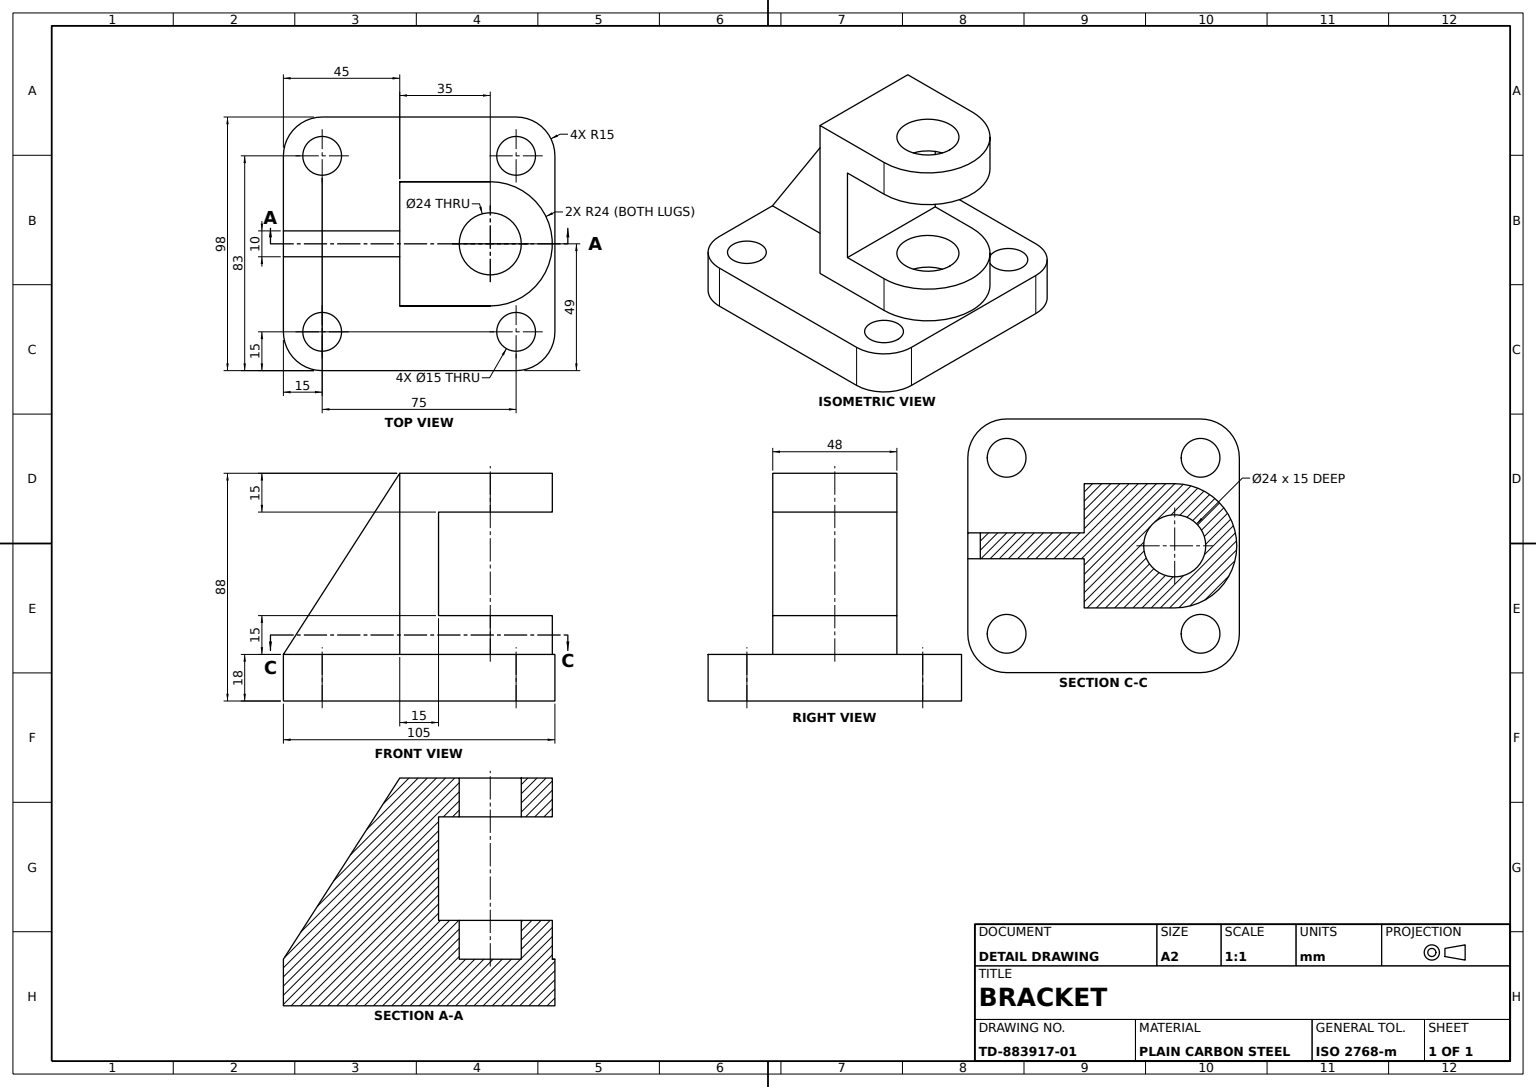
SolidWorks part; units mm, degrees
material "Plain Carbon Steel"
ref_plane "Front Plane" through (0, 0, 0) normal (0, 0, 1) x (1, 0, 0)
ref_plane "Top Plane" through (0, 0, 0) normal (0, 1, 0) x (1, 0, 0)
ref_plane "Right Plane" through (0, 0, 0) normal (1, 0, 0) x (0, 0, -1)
sketch "Base Plate Sketch" plane through (0, 0, 0) normal (0, 1, 0) x (1, 0, 0)
  line L1 (-34, -52.5) -> (34, -52.5)
  line L2 (-49, -37.5) -> (-49, 37.5)
  line L3 (-34, 52.5) -> (34, 52.5)
  line L4 (49, -37.5) -> (49, 37.5)
  line L5 (-49, -52.5) -> (49, 52.5) construction
  line L6 (-49, 52.5) -> (49, -52.5) construction
  arc A0 (-34, -52.5) -> (-49, -37.5) centre (-34, -37.5) cw
  arc A1 (34, -52.5) -> (49, -37.5) centre (34, -37.5) ccw
  arc A2 (34, 52.5) -> (49, 37.5) centre (34, 37.5) cw
  arc A3 (-49, 37.5) -> (-34, 52.5) centre (-34, 37.5) cw
  point P0 (0, 0)
  dimension "D3" = 15
  dimension "D1" = 98
  dimension "D2" = 105
extrude "Base Plate" add sketch "Base Plate Sketch" along normal blind 18
sketch "Mounting Holes Sketch" plane through (0, 18, 0) normal (0, 1, 0) x (1, 0, 0)
  line L0 (49, -37.5) -> (49, 37.5) construction
  circle A0 centre (-34, 37.5) radius 7.5
  circle A1 centre (34, 37.5) radius 7.5
  circle A2 centre (-34, -37.5) radius 7.5
  circle A3 centre (34, -37.5) radius 7.5
  dimension "D2" = 15
  dimension "D1" = 15
  dimension "D3" = 83
  dimension "D4" = 75
extrude "Mounting Holes 4xØ15" cut sketch "Mounting Holes Sketch" against normal blind 18
sketch "Upright Column Sketch" plane through (0, 0, 0) normal (0, 0, 1) x (1, 0, 0)
  line L0 (0, 0) -> (0, 55.5407) construction
  line L1 (-34, 18) -> (34, 18) construction
  line L2 (-24, 18) -> (24, 18)
  line L3 (-24, 18) -> (-24, 88)
  line L4 (-24, 88) -> (24, 88)
  line L5 (24, 18) -> (24, 88)
  dimension "D1" = 24
  dimension "D2" = 70
  dimension "24" = 24
extrude "Upright Column" add sketch "Upright Column Sketch" along normal mid plane 15
sketch "Support Rib Sketch" plane through (0, 0, 0) normal (1, 0, 0) x (0, 0, -1)
  line L0 (-7.5, 88) -> (-52.5, 18)
rib "Support Rib" sketch "Support Rib Sketch" sketch "Support Rib Sketch" thickness 10 extrusion direction parallel to sketch draft on no parameters "D1"=10
sketch "Clevis Lug 1 Sketch" plane through (0, 88, 0) normal (0, 1, 0) x (1, 0, 0)
  line L0 (-24, -7.5) -> (-24, 27.5)
  line L1 (24, 27.5) -> (24, -7.5)
  line L2 (0, -7.5) -> (0, 59.9792) construction
  line L3 (5, -7.5) -> (-5, -7.5) construction
  line L4 (-24, -7.5) -> (24, -7.5)
  arc A0 (-24, 27.5) -> (24, 27.5) centre (0, 27.5) cw
  circle A1 centre (0, 27.5) radius 12
  dimension "D2" = 24
  dimension "D1" = 35
extrude "Clevis Lug 1" add sketch "Clevis Lug 1 Sketch" against normal blind 15
sketch "Clevis Lug 2 Sketch" plane through (0, 18, 0) normal (0, 1, 0) x (1, 0, 0)
  line L1 (-24, -7.5) -> (24, -7.5)
  line L2 (-24, -7.5) -> (-24, 27.5)
  line L3 (24, 27.5) -> (24, -7.5)
  line L12 (34, 52.5) -> (-34, 52.5)
  line L13 (-49, 37.5) -> (-49, -37.5)
  line L14 (-34, -52.5) -> (-5, -52.5)
  line L15 (-5, -52.5) -> (-5, -7.5)
  line L16 (-5, -7.5) -> (-24, -7.5)
  line L17 (-24, -7.5) -> (-24, 7.5)
  line L18 (-24, 7.5) -> (24, 7.5)
  line L19 (24, 7.5) -> (24, -7.5)
  line L20 (24, -7.5) -> (5, -7.5)
  line L21 (5, -7.5) -> (5, -52.5)
  line L22 (5, -52.5) -> (34, -52.5)
  line L23 (49, -37.5) -> (49, 37.5)
  line L28 (-5, -7.5) -> (-24, -7.5)
  line L29 (-24, -7.5) -> (-24, 7.5)
  line L31 (24, 7.5) -> (24, -7.5)
  line L32 (24, -7.5) -> (5, -7.5)
  arc A0 (-24, 27.5) -> (24, 27.5) centre (0, 27.5) cw
  circle A1 centre (0, 27.5) radius 12
  arc A4 (-34, 52.5) -> (-49, 37.5) centre (-34, 37.5) ccw
  arc A5 (-49, -37.5) -> (-34, -52.5) centre (-34, -37.5) ccw
  arc A6 (34, -52.5) -> (49, -37.5) centre (34, -37.5) ccw
  arc A7 (49, 37.5) -> (34, 52.5) centre (34, 37.5) ccw
  line M28 (-24, 7.5) -> (24, 7.5)
  dimension "D2" = 24
  dimension "D1" = 0
extrude "Clevis Lug 2" add sketch "Clevis Lug 2 Sketch" along normal blind 15 contours A0 L2 L3 A1 M28
